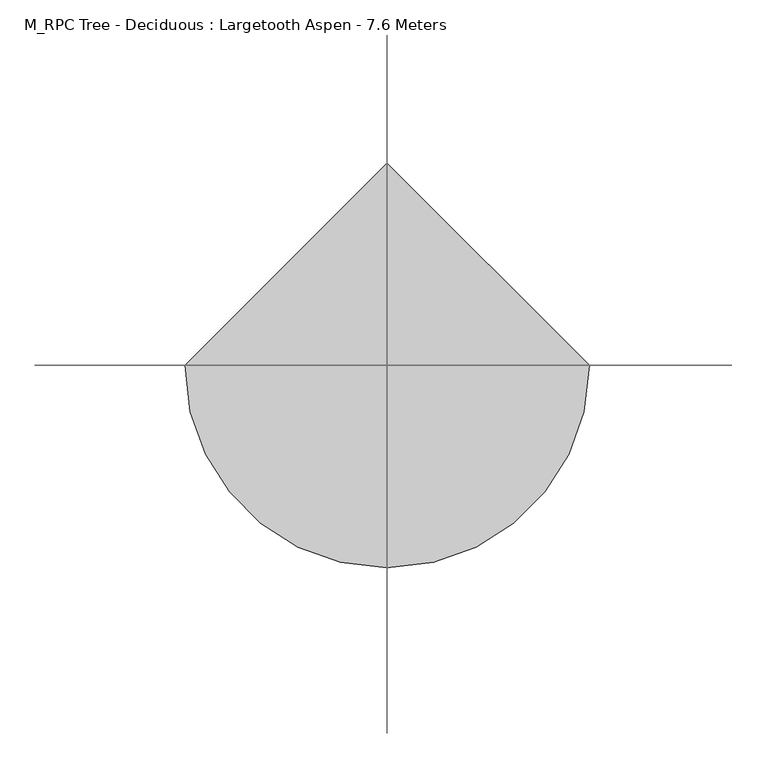
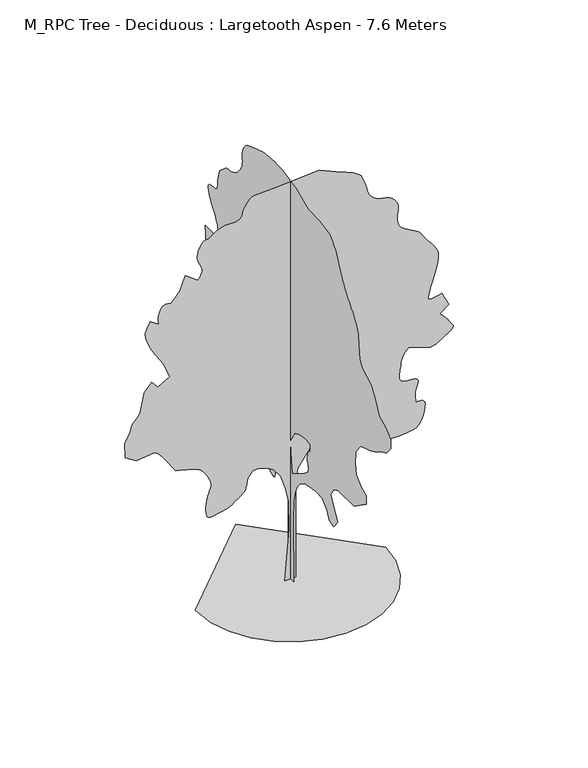
"""IFC4 building model written with IfcOpenShell, lengths in millimetres: geographic element geometry, M_RPC Tree - Deciduous : Largetooth Aspen - 7.6 Meters."""

from ifc_helpers import new_model, si_unit, origin, place, context, project, spatial, triangles, source, transform, mapped, element, save


def m_rpc_tree_deciduous_largetooth_aspen_7_6_meters_a2efc43f(model_context):
    return source(origin(), model_context, "Body", "Tessellation", [
        triangles([(92.8617737, 0.000406, 0.005513), (-103.915959, 0.000406, 0.005513), (-22.8901635, 0.0003494, 949.1680813), (-34.4652064, 0.0003176, 1481.626133), (-92.3406663, 0.0003011, 1759.4311237), (-173.3674883, 0.0002866, 2002.5093098), (-300.6936918, 0.0002762, 2176.1362118), (-404.8693279, 0.0002728, 2234.0127663), (-566.9214277, 0.0002694, 2291.8891754), (-682.6743914, 0.0002694, 2291.8891754), (-763.7004049, 0.0002762, 2176.1362118), (-798.427355, 0.0002852, 2025.6589142), (-801.2950579, 0.0002863, 2008.1460297), (-806.4934324, 0.0002874, 1989.7185207), (-816.3455927, 0.0002886, 1969.4722275), (-833.1871519, 0.0002899, 1946.489764), (-859.3387533, 0.0002915, 1919.8644997), (-897.1360102, 0.0002934, 1888.6816647), (-948.9046526, 0.0002956, 1852.0320122), (-998.3097038, 0.0002977, 1817.003627), (-1032.3247061, 0.0002993, 1790.0718407), (-1058.2431822, 0.0003005, 1769.4200489), (-1083.3510246, 0.0003015, 1753.2219097), (-1114.9365967, 0.0003023, 1739.6560226), (-1160.2933485, 0.000303, 1726.8980804), (-1226.7072453, 0.0003038, 1713.1294441), (-1299.8367931, 0.0003048, 1697.5064152), (-1361.0192505, 0.0003056, 1683.0943588), (-1411.0653236, 0.0003062, 1673.9514576), (-1450.7852829, 0.0003062, 1674.1187439), (-1480.9902706, 0.0003054, 1687.6517841), (-1502.4856155, 0.0003035, 1718.5964069), (-1516.0869656, 0.0003004, 1771.0059986), (-1522.0251205, 0.0002967, 1833.4043701), (-1521.0802654, 0.0002932, 1891.7521168), (-1514.8710514, 0.00029, 1946.2541679), (-1505.0164204, 0.0002869, 1997.1108021), (-1493.1376396, 0.0002841, 2044.5246231), (-1480.8535057, 0.0002815, 2088.6983803), (-1469.7852859, 0.000279, 2129.8370029), (-1458.1775642, 0.0002769, 2165.8103886), (-1444.9485752, 0.000275, 2196.5194153), (-1432.7328964, 0.0002733, 2225.2042923), (-1424.1600185, 0.0002715, 2255.1052288), (-1421.8648098, 0.0002695, 2289.4596725), (-1428.479377, 0.000267, 2331.5079781), (-1446.6356815, 0.0002638, 2384.4900639), (-1473.3978561, 0.0002604, 2441.7913628), (-1503.3976238, 0.0002573, 2494.2338013), (-1535.6266159, 0.0002545, 2541.2094223), (-1569.0690514, 0.0002521, 2582.1226227), (-1602.7142361, 0.00025, 2616.3228607), (-1635.5487144, 0.0002484, 2643.2520309), (-1666.5642632, 0.0002473, 2662.3026123), (-1701.7269424, 0.0002464, 2677.1732162), (-1746.6125748, 0.0002455, 2692.0694), (-1799.5946606, 0.0002446, 2706.940004), (-1859.0568741, 0.0002437, 2721.8358971), (-1923.3782387, 0.0002428, 2736.706501), (-1990.9396671, 0.000242, 2751.5771049), (-2060.1197468, 0.0002411, 2766.4732887), (-2256.8962532, 0.0002238, 3055.8556252), (-2301.7818855, 0.0002202, 3116.5289566), (-2338.160479, 0.0002175, 3161.4195305), (-2367.4508423, 0.0002156, 3193.1367805), (-2391.0741096, 0.0002144, 3214.3154297), (-2410.4440029, 0.0002136, 3227.61549), (-2426.9815109, 0.0002131, 3235.6461044), (-2442.1003555, 0.0002128, 3241.041996), (-2766.1945267, 0.0002148, 3206.3353935), (-2962.9836777, 0.0002073, 3333.6607613), (-2974.5611687, 0.0001914, 3599.8884064), (-2952.3436295, 0.000189, 3639.5351143), (-2930.8609291, 0.0001867, 3678.9789276), (-2910.7717484, 0.0001843, 3718.0428223), (-2892.8103447, 0.0001821, 3756.473616), (-2877.7118477, 0.0001798, 3794.0934128), (-2866.1343567, 0.0001776, 3830.70019), (-2858.8130013, 0.0001755, 3866.1160515), (-2847.3878265, 0.0001735, 3899.5814507), (-2825.6772331, 0.0001716, 3931.2481224), (-2797.4559906, 0.0001698, 3962.0787987), (-2766.6000252, 0.0001679, 3993.137368), (-2736.9852631, 0.000166, 4025.3865623), (-2712.4120537, 0.000164, 4059.8905609), (-2696.7560326, 0.0001617, 4097.611805), (-2627.2919586, 0.000141, 4444.881015), (-2488.4021805, 0.0001321, 4595.3354942), (-2384.2239464, 0.0001396, 4468.0101265), (-2164.2953648, 0.0001327, 4583.7832924), (-2280.0483284, 0.0001155, 4873.1403397), (-2465.2501053, 9.82e-05, 5162.5226761), (-2487.5231644, 9.58e-05, 5203.6643509), (-2513.036142, 9.27e-05, 5254.9385468), (-2539.3601166, 8.93e-05, 5312.268187), (-2564.0600624, 8.58e-05, 5371.6238663), (-2584.7067673, 8.24e-05, 5428.9535065), (-2598.8934013, 7.93e-05, 5480.2277023), (-2604.1628471, 7.69e-05, 5521.3693771), (-2601.4519661, 7.48e-05, 5555.7463486), (-2593.9027176, 7.28e-05, 5589.5407974), (-2582.2746483, 7.08e-05, 5622.8038834), (-2567.4293335, 6.89e-05, 5655.6611801), (-2550.1521904, 6.69e-05, 5688.2394241), (-2531.2585762, 6.5e-05, 5720.5903564), (-2511.5516396, 6.31e-05, 5752.8651306), (-2361.0744873, 6.93e-05, 5648.6941635), (-2365.8675087, 6.73e-05, 5681.019516), (-2369.6472198, 6.54e-05, 5713.8518143), (-2371.4003105, 6.34e-05, 5747.6968414), (-2370.118412, 6.13e-05, 5783.0621246), (-2364.7857433, 5.9e-05, 5820.4540283), (-2354.391465, 5.67e-05, 5860.3794983), (-2337.9248829, 5.41e-05, 5903.344899), (-2316.394075, 5.19e-05, 5940.9141174), (-2291.8258072, 5.04e-05, 5965.7155106), (-2264.7267345, 4.95e-05, 5979.8768555), (-2235.6036575, 4.92e-05, 5985.5515091), (-2204.9604698, 4.92e-05, 5984.8422501), (-2173.3064426, 4.95e-05, 5979.8768555), (-2141.1459057, 5e-05, 5972.7831024), (-1990.6686081, 3.96e-05, 6146.4178528), (-1886.4928448, 2.44e-05, 6401.0680069), (-1666.5642632, 3.41e-05, 6239.0110382), (-1644.4939533, 3.23e-05, 6268.8284042), (-1623.9409927, 3.05e-05, 6298.823085), (-1606.4256374, 2.87e-05, 6329.2229736), (-1593.4675621, 2.69e-05, 6360.2309647), (-1586.584552, 2.5e-05, 6392.0749512), (-1587.2913403, 2.3e-05, 6424.9066681), (-1597.1131245, 2.1e-05, 6458.9545898), (-1613.1085144, 1.89e-05, 6493.7879288), (-1630.1173599, 1.68e-05, 6529.2043716), (-1646.3153538, 1.46e-05, 6565.8614365), (-1659.8813862, 1.23e-05, 6604.3428085), (-1668.993766, 9.9e-06, 6645.2304291), (-1671.8286221, 7.3e-06, 6689.1585617), (-1666.5642632, 4.4e-06, 6736.759726), (-1653.9432312, 1.5e-06, 6785.3747818), (-1636.4607227, -1.2e-06, 6830.974324), (-1614.9299149, -3.6e-06, 6871.9131042), (-1590.1616592, -5.7e-06, 6906.5691284), (-1562.9612846, -7.3e-06, 6933.3209839), (-1534.1394974, -8.3e-06, 6950.5728378), (-1504.512236, -8.7e-06, 6956.6782791), (-1471.3382435, -9.2e-06, 6965.0132355), (-1431.8891979, -1.05e-05, 6986.521225), (-1386.9707188, -1.22e-05, 7015.9078033), (-1337.3959831, -1.41e-05, 7047.9291046), (-1283.9756973, -1.59e-05, 7077.315683), (-1227.5178062, -1.72e-05, 7098.8236725), (-1168.8306908, -1.77e-05, 7107.1580475), (-1109.0314339, -1.76e-05, 7106.8289978), (-1050.4481638, -1.77e-05, 7107.2847839), (-995.7104439, -1.79e-05, 7110.8060806), (-947.4530697, -1.84e-05, 7119.5718246), (-908.3054592, -1.94e-05, 7135.8353668), (-880.9024807, -2.09e-05, 7161.8273849), (-867.8760956, -2.32e-05, 7199.7512329), (-856.9422426, -2.61e-05, 7248.5941818), (-835.6824938, -2.93e-05, 7302.6804153), (-806.5264246, -3.26e-05, 7357.4009125), (-771.9008492, -3.56e-05, 7408.0420074), (-734.2403572, -3.81e-05, 7449.9940979), (-695.9718355, -3.98e-05, 7478.5696793), (-659.5247869, -4.04e-05, 7489.1335693), (-323.8458215, -4.18e-05, 7512.2885513), (509.5693688, -4.53e-05, 7570.1751343), (926.2744205, -3.42e-05, 7384.9631836), (995.3532709, -3.26e-05, 7357.5526474), (1062.2078384, -3.09e-05, 7329.4578506), (1124.6038118, -2.92e-05, 7299.9195374), (1180.3219225, -2.73e-05, 7268.2778641), (1227.1277138, -2.52e-05, 7233.7741562), (1262.7970482, -2.29e-05, 7195.7485703), (1285.1055702, -2.04e-05, 7153.4674301), (1299.9533558, -1.79e-05, 7111.9461273), (1314.5985374, -1.58e-05, 7075.1117477), (1328.8409821, -1.37e-05, 7040.480722), (1342.4753242, -1.16e-05, 7005.6473831), (1355.2991055, -9.4e-06, 6968.1799026), (1367.1094311, -6.8e-06, 6925.6702881), (1377.7063133, -3.9e-06, 6875.662294), (1393.5345623, -8e-07, 6823.9573105), (1419.2834267, 2e-06, 6778.1292938), (1452.117905, 4.3e-06, 6738.3811386), (1489.2059029, 6.3e-06, 6704.890741), (1527.709948, 7.9e-06, 6677.9104111), (1564.7979458, 9.1e-06, 6657.5936279), (1597.6348949, 9.9e-06, 6644.1415421), (1628.0070236, 1.04e-05, 6636.0856384), (1659.1872425, 1.07e-05, 6630.6638763), (1690.5726814, 1.1e-05, 6626.230426), (1721.5527672, 1.13e-05, 6621.2144531), (1751.5195427, 1.17e-05, 6613.9439667), (1779.8675217, 1.24e-05, 6602.8481323), (1805.9861309, 1.34e-05, 6586.2799576), (1831.2638031, 1.47e-05, 6563.7586578), (1856.5388592, 1.63e-05, 6536.6015945), (1880.3977226, 1.82e-05, 6505.7959167), (1901.4218754, 2.02e-05, 6472.3560974), (1918.1949795, 2.23e-05, 6437.2948654), (1929.2986622, 2.44e-05, 6401.625531), (1933.3139694, 2.65e-05, 6366.3364059), (1929.8053173, 2.9e-05, 6325.1191544), (1922.2457497, 3.2e-05, 6273.1351181), (1915.0916805, 3.56e-05, 6213.8805954), (1912.7964718, 3.93e-05, 6150.775145), (1919.8163921, 4.31e-05, 6087.2644867), (1940.6048035, 4.67e-05, 6026.7937592), (1979.615649, 5e-05, 5972.7831024), (2034.2165314, 5.26e-05, 5927.5631882), (2096.1082478, 5.5e-05, 5888.8289246), (2161.2401733, 5.71e-05, 5853.1340103), (2225.5615379, 5.92e-05, 5817.0088898), (2285.0238968, 6.16e-05, 5777.0584213), (2335.5764797, 6.44e-05, 5729.8118866), (2373.1711327, 6.79e-05, 5671.8491455), (2411.6421856, 7.17e-05, 5607.223439), (2462.6659607, 7.56e-05, 5541.7878983), (2518.9567108, 7.96e-05, 5474.7303635), (2573.2307236, 8.38e-05, 5405.2410004), (2618.1721664, 8.81e-05, 5332.5093933), (2646.5201454, 9.27e-05, 5255.7495438), (2650.9785942, 9.76e-05, 5174.0998764), (2634.6386032, 0.0001032, 5079.7841217), (2608.190799, 0.0001097, 4970.8762344), (2575.6628426, 0.0001165, 4855.508567), (2541.0826859, 0.0001233, 4741.7367325), (2508.5622871, 0.0001295, 4637.6927925), (2482.1043091, 0.0001347, 4551.4835197), (2465.7718758, 0.0001383, 4491.1648178), (2464.9611694, 0.0001404, 4454.9635391), (2480.5538223, 0.0001417, 4433.9369156), (2509.8113388, 0.0001422, 4425.5769608), (2550.0001648, 0.0001421, 4427.3248192), (2598.3867462, 0.0001415, 4436.6727951), (2652.2453773, 0.0001407, 4451.0876129), (2708.839888, 0.0001396, 4468.0101265), (2836.1652557, 0.0001548, 4213.3596817), (2674.1332855, 0.0001624, 4086.0346046), (2698.8841003, 0.0001637, 4063.6400414), (2723.4573097, 0.0001651, 4040.7132431), (2747.6253113, 0.0001665, 4016.7987144), (2771.1852104, 0.0001681, 3991.3386406), (2793.9344032, 0.0001697, 3963.8772354), (2815.6705765, 0.0001715, 3933.8828453), (2836.1652557, 0.0001735, 3900.8482338), (2858.1037422, 0.0001754, 3868.6749069), (2881.2584335, 0.000177, 3840.554821), (2901.1702995, 0.0001786, 3814.8921432), (2913.3811821, 0.0001801, 3790.0148827), (2913.4570496, 0.0001816, 3764.3269157), (2896.9144547, 0.0001833, 3736.232119), (2859.3199471, 0.0001852, 3704.0590828), (2604.6695023, 0.0001955, 3530.4243324), (2500.4962097, 0.0001962, 3518.8471321), (2118.5182171, 0.0001886, 3646.1722092), (2091.3836815, 0.0001903, 3618.7110947), (2065.163625, 0.000192, 3590.1349319), (2040.7651142, 0.0001938, 3559.3298355), (2019.0975414, 0.0001958, 3525.1551773), (2001.0780018, 0.0001981, 3486.5726486), (1987.6134167, 0.0002008, 3442.3913338), (1979.615649, 0.0002038, 3391.5220551), (1974.0473843, 0.0002068, 3342.1474525), (1967.6684132, 0.0002092, 3301.2848305), (1961.0868382, 0.0002113, 3266.096862), (1954.9106163, 0.0002132, 3233.7206406), (1949.7477047, 0.0002151, 3201.3699989), (1946.2035896, 0.0002172, 3166.1567413), (1944.888699, 0.0002197, 3125.2941193), (1953.8643139, 0.000222, 3086.7368797), (1977.0163891, 0.0002236, 3059.0981598), (2008.6704163, 0.0002247, 3040.5542336), (2043.1591541, 0.0002254, 3029.3316628), (2074.8131813, 0.0002257, 3023.5555618), (2097.9652565, 0.0002259, 3021.4277847), (2106.9408714, 0.0002259, 3021.1237335), (2119.5973663, 0.0002258, 3022.0103073), (2151.4868443, 0.0002258, 3022.4663841), (2193.5021576, 0.000226, 3019.2997169), (2236.5307812, 0.0002266, 3009.2421913), (2271.4578644, 0.0002278, 2989.0771431), (2289.1759689, 0.0002298, 2955.5102966), (2280.5702442, 0.0002328, 2905.3758568), (2259.8146797, 0.0002362, 2847.8691925), (2246.3499493, 0.0002394, 2794.0105614), (2238.9578133, 0.0002425, 2743.191861), (2236.4270084, 0.0002453, 2694.7799904), (2237.5416206, 0.0002481, 2648.2174255), (2241.0857357, 0.0002508, 2602.8707748), (2245.8432941, 0.0002535, 2558.1066467), (2285.1910378, 0.0002532, 2562.540097), (2322.5171024, 0.0002531, 2563.730722), (2355.7899261, 0.0002535, 2558.4106979), (2382.9903008, 0.0002544, 2543.4133575), (2402.0916058, 0.000256, 2515.4278564), (2411.0672207, 0.0002587, 2471.2540993), (2407.8954666, 0.0002625, 2407.6395229), (2395.1731327, 0.0002668, 2334.9507912), (2376.9836906, 0.0002708, 2266.9155544), (2353.5301804, 0.0002745, 2205.3632069), (2325.0124443, 0.0002777, 2152.110062), (2291.6383186, 0.0002803, 2108.9801365), (2253.6054657, 0.0002821, 2077.7999176), (2211.1189602, 0.0002832, 2060.3858643), (2171.2620907, 0.0002837, 2051.7801395), (2137.4826118, 0.000284, 2045.4011684), (2104.5113686, 0.0002843, 2040.64361), (2067.0864727, 0.0002845, 2036.8967457), (2019.9412399, 0.0002847, 2033.5578506), (1957.8137821, 0.000285, 2030.0137356), (1875.4374149, 0.0002852, 2025.6589142), (1785.9069786, 0.0002851, 2027.1105698), (1704.880965, 0.0002844, 2040.1039627), (1630.9405655, 0.000283, 2062.7139198), (1562.6724941, 0.0002812, 2093.0175934), (1498.6551807, 0.0002791, 2129.0947517), (1437.4727234, 0.0002767, 2169.0176056), (1377.7063133, 0.0002742, 2210.8631618), (1123.0508543, 0.0002597, 2453.9412025), (856.8231365, 0.0002528, 2569.6841377), (544.2937391, 0.0002542, 2546.5547356), (393.8164052, 0.0002611, 2430.7917435), (289.6407691, 0.00027, 2280.3144459), (127.5871523, 0.0002838, 2048.8109894), (92.8617737, 0.0003011, 1759.4311237), (92.8617737, 0.0003383, 1134.3723289), (-0.0023646, 90.6053344, 1.1e-05), (-0.0023646, -94.5971056, 0.0), (-0.0023646, -83.0220672, 1157.5168465), (-0.0023646, -94.5971056, 1527.9227257), (-0.0023646, -140.8980313, 1724.6992321), (-0.0023646, -210.3490428, 1875.1765297), (-0.0023646, -302.9508941, 1990.9294933), (-0.0023646, -441.8534077, 2071.9555069), (-0.0023646, -557.6038279, 2095.1051113), (-0.0023646, -789.1072117, 2141.4067909), (-0.0023646, -985.8861889, 2129.8320614), (-0.0023646, -1136.3635592, 1979.3546185), (-0.0023646, -1205.8147705, 1840.4521957), (-0.0023646, -1333.1399929, 1794.1505161), (-0.0023646, -1472.042561, 1967.7774181), (-0.0023646, -1321.5652634, 2199.2832001), (-0.0023646, -1252.1139793, 2361.3353725), (-0.0023646, -1333.1399929, 2500.2354698), (-0.0023646, -1483.6172905, 2569.6841377), (-0.0023646, -1969.7736626, 2569.6841377), (-0.0023646, -2351.7542713, 2835.9117828), (-0.0023646, -2351.7542713, 2997.9690422), (-0.0023646, -2189.7022442, 3067.4075363), (-0.0023646, -2039.2249466, 3206.3101044), (-0.0023646, -2004.5004673, 3403.0992554), (-0.0023646, -2027.6500717, 3634.5950089), (-0.0023646, -2178.1273693, 3831.3841599), (-0.0023646, -2444.3551598, 3923.9773453), (-0.0023646, -2488.9367409, 3941.4068047), (-0.0023646, -2533.110498, 3959.1147354), (-0.0023646, -2576.4735489, 3977.4307686), (-0.0023646, -2618.6279526, 3996.6839539), (-0.0023646, -2659.1612343, 4017.1280548), (-0.0023646, -2697.6678955, 4039.0918304), (-0.0023646, -2733.7427284, 4062.8799133), (-0.0023646, -2768.4493309, 4086.3386559), (-0.0023646, -2803.1812225, 4107.3652794), (-0.0023646, -2837.9131142, 4126.3652824), (-0.0023646, -2872.6450058, 4143.7438728), (-0.0023646, -2907.351899, 4159.9065491), (-0.0023646, -2942.0837906, 4175.258519), (-0.0023646, -2976.8156822, 4190.2052811), (-0.0023646, -3104.1407593, 4352.2622498), (-0.0023646, -3104.1407593, 4514.3195091), (-0.0023646, -2953.6609909, 4653.2220772), (-0.0023646, -2756.8971291, 4757.3924629), (-0.0023646, -2629.5467628, 5000.4657074), (-0.0023646, -2502.234185, 5185.6776581), (-0.0023646, -2224.4290489, 5336.1574265), (-0.0023646, -2143.4030354, 5463.4827942), (-0.0023646, -2120.2509602, 5718.1329483), (-0.0023646, -2097.1013557, 5926.4743011), (-0.0023646, -2072.264645, 5978.4327576), (-0.0023646, -2047.225185, 6029.4540619), (-0.0023646, -2021.7779011, 6078.651059), (-0.0023646, -1995.7251308, 6125.1127579), (-0.0023646, -1968.8641251, 6167.9514221), (-0.0023646, -1940.9873383, 6206.2043198), (-0.0023646, -1911.8997242, 6239.0110382), (-0.0023646, -1875.8225658, 6277.7964615), (-0.0023646, -1830.2327614, 6330.9455429), (-0.0023646, -1779.7788643, 6393.0121033), (-0.0023646, -1729.1274502, 6458.4988037), (-0.0023646, -1682.9270725, 6521.9838821), (-0.0023646, -1645.83922, 6577.9705811), (-0.0023646, -1622.5198586, 6620.9865601), (-0.0023646, -1605.6807701, 6657.1372604), (-0.0023646, -1585.6016178, 6696.1255783), (-0.0023646, -1563.2930958, 6737.9253525), (-0.0023646, -1539.7736012, 6782.5877426), (-0.0023646, -1516.0490318, 6830.0627518), (-0.0023646, -1493.1350235, 6880.3742157), (-0.0023646, -1472.042561, 6933.5238785), (-0.0023646, -1448.8245014, 6986.749118), (-0.0023646, -1419.5316673, 7037.5425293), (-0.0023646, -1385.1770782, 7086.3087387), (-0.0023646, -1346.7743351, 7133.4541168), (-0.0023646, -1305.3316612, 7179.3832901), (-0.0023646, -1261.8673084, 7224.5020477), (-0.0023646, -1217.3895727, 7269.2155975), (-0.0023646, -893.2828297, 7327.0766006), (-0.0023646, -546.029062, 7338.653801), (-0.0023646, -175.623419, 7500.711351), (-0.0023646, 264.2314734, 7593.3045364), (-0.0023646, 323.6937959, 7595.7363647), (-0.0023646, 382.7508016, 7597.8641418), (-0.0023646, 440.9996807, 7599.3843979), (-0.0023646, 498.0300296, 7599.9925003), (-0.0023646, 553.4441254, 7599.3843979), (-0.0023646, 606.831528, 7597.2566208), (-0.0023646, 657.7895004, 7593.3045364), (-0.0023646, 706.7891258, 7588.2379852), (-0.0023646, 754.9781902, 7582.5883301), (-0.0023646, 802.9670488, 7575.6974716), (-0.0023646, 851.3612606, 7566.9828873), (-0.0023646, 900.7663118, 7555.8620544), (-0.0023646, 951.7900869, 7541.6751297), (-0.0023646, 1005.0432318, 7523.8657516), (-0.0023646, 1340.7248497, 7408.1181656), (-0.0023646, 1370.3545818, 7383.1138779), (-0.0023646, 1399.173753, 7356.8683868), (-0.0023646, 1426.3741276, 7328.2166473), (-0.0023646, 1451.1425285, 7295.9418732), (-0.0023646, 1472.6733364, 7258.7778625), (-0.0023646, 1490.1558449, 7215.5595703), (-0.0023646, 1502.7768768, 7165.019632), (-0.0023646, 1507.1292274, 7116.7342072), (-0.0023646, 1503.584967, 7077.7714691), (-0.0023646, 1497.0060081, 7043.2421814), (-0.0023646, 1492.2458336, 7008.3076859), (-0.0023646, 1494.1711521, 6968.128743), (-0.0023646, 1507.6358826, 6917.7916992), (-0.0023646, 1537.5012108, 6852.5078934), (-0.0023646, 1578.4019119, 6786.1851974), (-0.0023646, 1620.9238804, 6734.4546341), (-0.0023646, 1663.8485859, 6694.8587952), (-0.0023646, 1705.9652012, 6664.9908508), (-0.0023646, 1746.0576668, 6642.4189728), (-0.0023646, 1782.9075977, 6624.7107513), (-0.0023646, 1815.3063469, 6609.4093597), (-0.0023646, 1845.0703732, 6598.3135254), (-0.0023646, 1874.8345448, 6592.8923447), (-0.0023646, 1904.598571, 6590.2826202), (-0.0023646, 1934.3652134, 6587.6984756), (-0.0023646, 1964.129385, 6582.2522964), (-0.0023646, 1993.8934113, 6571.1558807), (-0.0023646, 2023.6575829, 6551.5483566), (-0.0023646, 2197.2869556, 6401.0680069), (-0.0023646, 2266.7357689, 6181.1500351), (-0.0023646, 2264.4760231, 6146.5445892), (-0.0023646, 2263.5310226, 6112.7751389), (-0.0023646, 2265.2182743, 6080.6021027), (-0.0023646, 2270.8549942, 6050.8858932), (-0.0023646, 2281.7533115, 6024.3875107), (-0.0023646, 2299.23582, 6001.9417877), (-0.0023646, 2324.612178, 5984.3608841), (-0.0023646, 2359.9116222, 5974.3033585), (-0.0023646, 2402.9047829, 5970.5285889), (-0.0023646, 2448.5301956, 5967.9700241), (-0.0023646, 2491.7284309, 5961.5605316), (-0.0023646, 2527.4306122, 5946.2341415), (-0.0023646, 2550.5826874, 5916.92314), (-0.0023646, 2556.1053154, 5868.6127167), (-0.0023646, 2547.4413094, 5812.448703), (-0.0023646, 2532.0893394, 5762.3651321), (-0.0023646, 2511.1641632, 5717.3475311), (-0.0023646, 2485.7878052, 5676.3837524), (-0.0023646, 2457.0700813, 5638.4599045), (-0.0023646, 2426.1228424, 5602.562677), (-0.0023646, 2394.0634621, 5567.6531799), (-0.0023646, 2369.3609001, 5525.4981949), (-0.0023646, 2345.2664406, 5483.4705276), (-0.0023646, 2322.3854244, 5441.6201752), (-0.0023646, 2301.3284248, 5400.0732925), (-0.0023646, 2282.698312, 5358.9321991), (-0.0023646, 2267.1081299, 5318.2974701), (-0.0023646, 2255.160894, 5278.2708435), (-0.0023646, 2248.95168, 5240.6254669), (-0.0023646, 2249.4254883, 5206.6025436), (-0.0023646, 2255.4649452, 5175.6201324), (-0.0023646, 2265.9605255, 5147.0695496), (-0.0023646, 2279.797617, 5120.3426926), (-0.0023646, 2295.861462, 5094.8320404), (-0.0023646, 2313.0374485, 5069.9294907), (-0.0023646, 2463.5147461, 5093.0844727), (-0.0023646, 2648.7240807, 5093.0844727), (-0.0023646, 2625.5693893, 4757.3924629), (-0.0023646, 2417.2130665, 4398.5716324), (-0.0023646, 2409.7574169, 4356.4422272), (-0.0023646, 2402.1979946, 4314.642453), (-0.0023646, 2394.4358231, 4273.4252014), (-0.0023646, 2386.3697456, 4233.1451019), (-0.0023646, 2377.898315, 4194.0559181), (-0.0023646, 2368.9227001, 4156.486409), (-0.0023646, 2359.3391281, 4120.7664963), (-0.0023646, 2344.9953815, 4082.1586784), (-0.0023646, 2323.9712288, 4037.2681046), (-0.0023646, 2299.5044083, 3988.3492882), (-0.0023646, 2274.8373093, 3937.5814568), (-0.0023646, 2253.2051994, 3887.2441223), (-0.0023646, 2237.8507587, 3839.5162216), (-0.0023646, 2232.0114349, 3796.6522682), (-0.0023646, 2236.7360012, 3758.6522621), (-0.0023646, 2249.9651356, 3723.6921867), (-0.0023646, 2270.279884, 3691.2656776), (-0.0023646, 2296.2641991, 3660.865789), (-0.0023646, 2326.5020336, 3631.9602859), (-0.0023646, 2359.5747242, 3604.0936729), (-0.0023646, 2394.0634621, 3576.7337151), (-0.0023646, 2706.5853745, 3646.1722092), (-0.0023646, 2723.8372284, 3596.6458717), (-0.0023646, 2740.3798233, 3547.4991623), (-0.0023646, 2755.5039001, 3499.1884483), (-0.0023646, 2768.4746201, 3452.0686501), (-0.0023646, 2778.6333023, 3406.5699738), (-0.0023646, 2785.245108, 3363.0979179), (-0.0023646, 2787.6266487, 3322.0832703), (-0.0023646, 2774.199852, 3282.9940865), (-0.0023646, 2739.6958534, 3244.7153183), (-0.0023646, 2692.8545265, 3206.6647339), (-0.0023646, 2642.3654572, 3168.1833618), (-0.0023646, 2596.9426483, 3128.7142593), (-0.0023646, 2565.3015564, 3087.5981644), (-0.0023646, 2556.1053154, 3044.2784248), (-0.0023646, 2564.4399811, 3002.6556747), (-0.0023646, 2578.8547989, 2966.5049744), (-0.0023646, 2598.3361679, 2934.9397499), (-0.0023646, 2621.8454887, 2906.9969788), (-0.0023646, 2648.4200294, 2881.7903778), (-0.0023646, 2676.9959015, 2858.3825043), (-0.0023646, 2706.5853745, 2835.9117828), (-0.0023646, 2776.0491577, 2604.4160294), (-0.0023646, 2709.3974121, 2602.1106468), (-0.0023646, 2644.670549, 2600.945311), (-0.0023646, 2583.7946136, 2601.984201), (-0.0023646, 2528.6796638, 2606.3667824), (-0.0023646, 2481.2656975, 2615.2081032), (-0.0023646, 2443.468586, 2629.6226303), (-0.0023646, 2417.2130665, 2650.725412), (-0.0023646, 2391.9710026, 2676.8694557), (-0.0023646, 2357.0109272, 2705.4453278), (-0.0023646, 2313.9494568, 2736.0478203), (-0.0023646, 2264.407568, 2768.2973053), (-0.0023646, 2210.0068188, 2801.7371246), (-0.0023646, 2152.3684765, 2835.987941), (-0.0023646, 2093.1088669, 2870.6436745), (-0.0023646, 2090.6463718, 2833.3785072), (-0.0023646, 2088.2828533, 2795.8345779), (-0.0023646, 2086.1244095, 2757.6572571), (-0.0023646, 2084.2675461, 2718.5680733), (-0.0023646, 2082.8158905, 2678.2879738), (-0.0023646, 2081.8710354, 2636.4626198), (-0.0023646, 2081.533992, 2592.838829), (-0.0023646, 2079.9481876, 2547.390731), (-0.0023646, 2074.514217, 2502.7332825), (-0.0023646, 2064.2212406, 2462.5418404), (-0.0023646, 2048.0560936, 2430.4471424), (-0.0023646, 2025.0077911, 2410.0994019), (-0.0023646, 1994.0631683, 2405.1366234), (-0.0023646, 1954.2062988, 2419.2093109), (-0.0023646, 1909.2219807, 2445.3635284), (-0.0023646, 1863.6321762, 2473.9469582), (-0.0023646, 1817.5331005, 2504.5546829), (-0.0023646, 1771.028817, 2536.7762627), (-0.0023646, 1724.222953, 2570.216082), (-0.0023646, 1677.2144852, 2604.4921875), (-0.0023646, 1630.1020992, 2639.147921), (-0.0023646, 1352.2995792, 2720.1639061), (-0.0023646, 1074.4945158, 2627.5707207), (-0.0023646, 900.8676138, 2419.2093109), (-0.0023646, 923.2419748, 2389.5794334), (-0.0023646, 945.9203871, 2360.7602623), (-0.0023646, 969.204213, 2333.5598877), (-0.0023646, 993.4000471, 2308.7914867), (-0.0023646, 1018.8119408, 2287.2608242), (-0.0023646, 1045.7412563, 2269.7783157), (-0.0023646, 1074.4945158, 2257.1571384), (-0.0023646, 1101.897567, 2244.8731499), (-0.0023646, 1125.0471714, 2228.3379673), (-0.0023646, 1144.6551315, 2208.258815), (-0.0023646, 1161.4257648, 2185.344952), (-0.0023646, 1176.07349, 2160.305492), (-0.0023646, 1189.3025517, 2133.8473686), (-0.0023646, 1201.8222816, 2106.6798409), (-0.0023646, 1169.4919149, 2099.1888737), (-0.0023646, 1136.6573639, 2091.3937099), (-0.0023646, 1102.8070318, 2082.9907345), (-0.0023646, 1067.4417486, 2073.6756054), (-0.0023646, 1030.0497723, 2063.1471783), (-0.0023646, 990.1269911, 2051.0986404), (-0.0023646, 947.16675, 2037.2285568), (-0.0023646, 904.2091249, 2020.3237747), (-0.0023646, 864.2863438, 1999.7708141), (-0.0023646, 826.8943674, 1976.1830097), (-0.0023646, 791.5265408, 1950.1630863), (-0.0023646, 757.6786795, 1922.3217625), (-0.0023646, 724.8442011, 1893.2645245), (-0.0023646, 692.5138344, 1863.6018002), (-0.0023646, 692.5138344, 1701.5496277), (-0.0023646, 650.5998957, 1674.7216141), (-0.0023646, 610.2059223, 1650.6246838), (-0.0023646, 572.8469018, 1631.9970417), (-0.0023646, 540.0453429, 1621.5699165), (-0.0023646, 513.3187039, 1622.0765717), (-0.0023646, 494.1844431, 1636.2505611), (-0.0023646, 484.160055, 1666.8252937), (-0.0023646, 479.2682024, 1701.4811726), (-0.0023646, 474.7791232, 1728.6487003), (-0.0023646, 471.100714, 1752.1706657), (-0.0023646, 468.638328, 1775.8927643), (-0.0023646, 467.7947385, 1803.6682491), (-0.0023646, 468.9752624, 1839.3374382), (-0.0023646, 472.5852528, 1886.7512592), (-0.0023646, 475.5213744, 1938.6212036), (-0.0023646, 474.8120427, 1985.6298168), (-0.0023646, 471.0677945, 2028.5899853), (-0.0023646, 464.8915363, 2068.3100899), (-0.0023646, 456.893805, 2105.6006916), (-0.0023646, 447.6800869, 2141.2724968), (-0.0023646, 437.8608825, 2176.1311249), (-0.0023646, 241.0823958, 2187.7059998), (-0.0023646, 136.90626, 1990.9294933), (-0.0023646, 79.030296, 1655.2479481), (-0.0023646, 79.030296, 1226.9681305), (-0.0023646, 79.030296, 590.3344608), (-0.0022449, -48.2969385, 2025.6538273), (-0.0022449, -1.9959556, 2396.0597065), (-0.0022449, 9.5791312, 2615.9935204), (-0.0022449, -129.3229929, 2835.9117828), (-0.0022449, -279.801326, 2905.3758568), (-0.0022449, -453.4282099, 2928.5049683), (-0.0022449, -615.4803097, 2928.5049683), (-0.0022449, -615.4803097, 2789.62798), (-0.0022449, -534.4542598, 2720.1639061), (-0.0022449, -511.3046917, 2558.1066467), (-0.0022449, -521.1568156, 2548.0241226), (-0.0022449, -530.6061298, 2536.9279976), (-0.0022449, -539.2448104, 2523.7927528), (-0.0022449, -546.6699749, 2507.6277512), (-0.0022449, -552.4738358, 2487.4115433), (-0.0022449, -556.2535832, 2462.1366325), (-0.0022449, -557.6038279, 2430.7840405), (-0.0022449, -554.2294335, 2398.4207542), (-0.0022449, -544.7801193, 2370.3109875), (-0.0022449, -530.2691955, 2345.7427197), (-0.0022449, -511.7075014, 2324.0093079), (-0.0022449, -490.1108545, 2304.4038185), (-0.0022449, -466.4875508, 2286.2145218), (-0.0022449, -441.8534077, 2268.7320133), (-1707.3661331, 0.0, 0.0031185), (-1662.2297894, -391.2146745, 0.0030952), (-1533.678479, -750.4840605, 0.0030738), (-1332.01012, -1067.5126745, 0.0030549), (-1067.5126745, -1332.01012, 0.0030391), (-750.4840605, -1533.678479, 0.0030271), (-391.2146745, -1662.2297894, 0.0030194), (7.48e-05, -1707.3661331, 0.0030167), (391.2146745, -1662.2297894, 0.0030194), (750.4840605, -1533.678479, 0.0030271), (1067.5126745, -1332.01012, 0.0030391), (1332.01012, -1067.5126745, 0.0030549), (1533.678479, -750.4840605, 0.0030738), (1662.2297894, -391.2146745, 0.0030952), (1707.3661331, 0.0001493, 0.0031185), (-0.0002245, 1707.3661331, 0.0032203)], [[122, 123, 124], [87, 88, 89], [1, 2, 3], [329, 1, 3], [329, 3, 4], [328, 329, 4], [328, 4, 5], [105, 106, 107], [327, 328, 5], [327, 5, 6], [104, 105, 107], [238, 239, 240], [238, 240, 241], [237, 238, 241], [236, 237, 241], [103, 104, 107], [86, 87, 89], [235, 236, 241], [102, 103, 107], [101, 102, 107], [100, 101, 107], [99, 100, 107], [98, 99, 107], [97, 98, 107], [96, 97, 107], [327, 6, 7], [326, 327, 7], [95, 96, 107], [70, 71, 72], [69, 70, 72], [69, 72, 73], [69, 73, 74], [69, 74, 75], [69, 75, 76], [69, 76, 77], [69, 77, 78], [94, 95, 107], [234, 235, 241], [93, 94, 107], [69, 78, 79], [69, 79, 80], [69, 80, 81], [69, 81, 82], [69, 82, 83], [69, 83, 84], [69, 84, 85], [68, 69, 85], [325, 326, 7], [325, 7, 8], [67, 68, 85], [92, 93, 107], [91, 92, 107], [60, 61, 62], [67, 85, 86], [67, 86, 89], [67, 89, 90], [66, 67, 90], [65, 66, 90], [64, 65, 90], [63, 64, 90], [62, 63, 90], [60, 62, 90], [59, 60, 90], [58, 59, 90], [57, 58, 90], [56, 57, 90], [55, 56, 90], [54, 55, 90], [53, 54, 90], [284, 285, 286], [283, 284, 286], [282, 283, 286], [282, 286, 287], [281, 282, 287], [280, 281, 287], [279, 280, 287], [279, 287, 288], [278, 279, 288], [277, 278, 288], [277, 288, 289], [276, 277, 289], [275, 276, 289], [275, 289, 290], [52, 53, 90], [325, 8, 9], [121, 122, 124], [275, 290, 291], [30, 31, 32], [29, 30, 32], [29, 32, 33], [28, 29, 33], [28, 33, 34], [27, 28, 34], [27, 34, 35], [27, 35, 36], [26, 27, 36], [26, 36, 37], [26, 37, 38], [25, 26, 38], [25, 38, 39], [24, 25, 39], [23, 24, 39], [22, 23, 39], [21, 22, 39], [20, 21, 39], [20, 39, 40], [20, 40, 41], [20, 41, 42], [19, 20, 42], [19, 42, 43], [18, 19, 43], [18, 43, 44], [17, 18, 44], [16, 17, 44], [15, 16, 44], [14, 15, 44], [13, 14, 44], [12, 13, 44], [11, 12, 44], [11, 44, 45], [11, 45, 46], [10, 11, 46], [10, 46, 47], [10, 47, 48], [10, 48, 49], [10, 49, 50], [10, 50, 51], [252, 253, 254], [251, 252, 254], [251, 254, 255], [250, 251, 255], [249, 250, 255], [249, 255, 256], [248, 249, 256], [247, 248, 256], [246, 247, 256], [245, 246, 256], [245, 256, 257], [245, 257, 258], [244, 245, 258], [243, 244, 258], [242, 243, 258], [241, 242, 258], [234, 241, 258], [233, 234, 258], [274, 275, 291], [324, 325, 9], [51, 52, 90], [10, 51, 90], [9, 10, 90], [324, 9, 90], [323, 324, 90], [323, 90, 91], [323, 91, 107], [323, 107, 108], [323, 108, 109], [323, 109, 110], [323, 110, 111], [323, 111, 112], [323, 112, 113], [323, 113, 114], [323, 114, 115], [323, 115, 116], [323, 116, 117], [323, 117, 118], [323, 118, 119], [323, 119, 120], [323, 120, 121], [323, 121, 124], [323, 124, 125], [323, 125, 126], [323, 126, 127], [323, 127, 128], [323, 128, 129], [322, 323, 129], [322, 129, 130], [167, 168, 169], [274, 291, 292], [296, 297, 298], [296, 298, 299], [295, 296, 299], [294, 295, 299], [294, 299, 300], [293, 294, 300], [293, 300, 301], [293, 301, 302], [293, 302, 303], [293, 303, 304], [293, 304, 305], [293, 305, 306], [293, 306, 307], [293, 307, 308], [293, 308, 309], [293, 309, 310], [293, 310, 311], [293, 311, 312], [293, 312, 313], [293, 313, 314], [293, 314, 315], [293, 315, 316], [293, 316, 317], [293, 317, 318], [293, 318, 319], [292, 293, 319], [274, 292, 319], [274, 319, 320], [274, 320, 321], [274, 321, 322], [273, 274, 322], [273, 322, 130], [272, 273, 130], [271, 272, 130], [270, 271, 130], [269, 270, 130], [268, 269, 130], [267, 268, 130], [266, 267, 130], [265, 266, 130], [264, 265, 130], [263, 264, 130], [262, 263, 130], [261, 262, 130], [260, 261, 130], [259, 260, 130], [258, 259, 130], [233, 258, 130], [232, 233, 130], [231, 232, 130], [230, 231, 130], [229, 230, 130], [228, 229, 130], [227, 228, 130], [226, 227, 130], [225, 226, 130], [224, 225, 130], [223, 224, 130], [222, 223, 130], [221, 222, 130], [220, 221, 130], [219, 220, 130], [218, 219, 130], [217, 218, 130], [216, 217, 130], [215, 216, 130], [214, 215, 130], [213, 214, 130], [212, 213, 130], [211, 212, 130], [210, 211, 130], [209, 210, 130], [208, 209, 130], [207, 208, 130], [206, 207, 130], [205, 206, 130], [204, 205, 130], [203, 204, 130], [202, 203, 130], [201, 202, 130], [200, 201, 130], [199, 200, 130], [198, 199, 130], [197, 198, 130], [196, 197, 130], [195, 196, 130], [194, 195, 130], [193, 194, 130], [192, 193, 130], [191, 192, 130], [190, 191, 130], [189, 190, 130], [188, 189, 130], [187, 188, 130], [186, 187, 130], [185, 186, 130], [184, 185, 130], [183, 184, 130], [182, 183, 130], [181, 182, 130], [180, 181, 130], [179, 180, 130], [178, 179, 130], [177, 178, 130], [176, 177, 130], [175, 176, 130], [174, 175, 130], [173, 174, 130], [172, 173, 130], [171, 172, 130], [170, 171, 130], [169, 170, 130], [167, 169, 130], [167, 130, 131], [167, 131, 132], [167, 132, 133], [167, 133, 134], [167, 134, 135], [167, 135, 136], [164, 165, 166], [164, 166, 167], [163, 164, 167], [162, 163, 167], [161, 162, 167], [160, 161, 167], [159, 160, 167], [158, 159, 167], [143, 144, 145], [142, 143, 145], [141, 142, 145], [140, 141, 145], [140, 145, 146], [139, 140, 146], [138, 139, 146], [137, 138, 146], [136, 137, 146], [136, 146, 147], [136, 147, 148], [136, 148, 149], [136, 149, 150], [136, 150, 151], [136, 151, 152], [136, 152, 153], [136, 153, 154], [136, 154, 155], [136, 155, 156], [157, 158, 167], [157, 167, 136], [157, 136, 156], [634, 330, 635], [633, 634, 635], [632, 633, 635], [631, 632, 635], [540, 541, 542], [592, 593, 594], [494, 495, 496], [635, 330, 331], [635, 331, 332], [635, 332, 333], [635, 333, 334], [635, 334, 335], [658, 635, 335], [658, 335, 336], [658, 336, 337], [658, 337, 338], [540, 542, 543], [657, 658, 338], [631, 635, 636], [630, 631, 636], [518, 519, 520], [656, 657, 338], [656, 338, 339], [655, 656, 339], [654, 655, 339], [653, 654, 339], [540, 543, 544], [539, 540, 544], [518, 520, 521], [539, 544, 545], [538, 539, 545], [538, 545, 546], [538, 546, 547], [538, 547, 548], [537, 538, 548], [537, 548, 549], [536, 537, 549], [536, 549, 550], [536, 550, 551], [535, 536, 551], [535, 551, 552], [534, 535, 552], [493, 494, 496], [493, 496, 497], [343, 344, 345], [342, 343, 345], [341, 342, 345], [340, 341, 345], [340, 345, 346], [534, 552, 553], [533, 534, 553], [518, 521, 522], [350, 351, 352], [349, 350, 352], [349, 352, 353], [348, 349, 353], [533, 553, 554], [652, 653, 339], [518, 522, 523], [518, 523, 524], [533, 554, 555], [532, 533, 555], [518, 524, 525], [518, 525, 526], [518, 526, 527], [518, 527, 528], [518, 528, 529], [518, 529, 530], [518, 530, 531], [518, 531, 532], [518, 532, 555], [517, 518, 555], [516, 517, 555], [515, 516, 555], [607, 608, 609], [591, 592, 594], [591, 594, 595], [590, 591, 595], [590, 595, 596], [589, 590, 596], [588, 589, 596], [588, 596, 597], [587, 588, 597], [586, 587, 597], [586, 597, 598], [585, 586, 598], [585, 598, 599], [584, 585, 599], [584, 599, 600], [583, 584, 600], [583, 600, 601], [582, 583, 601], [514, 515, 555], [643, 644, 645], [630, 636, 637], [629, 630, 637], [581, 582, 601], [581, 601, 602], [348, 353, 354], [580, 581, 602], [580, 602, 603], [579, 580, 603], [651, 652, 339], [651, 339, 340], [651, 340, 346], [650, 651, 346], [649, 650, 346], [649, 346, 347], [648, 649, 347], [647, 648, 347], [646, 647, 347], [372, 373, 374], [371, 372, 374], [370, 371, 374], [369, 370, 374], [369, 374, 375], [368, 369, 375], [367, 368, 375], [366, 367, 375], [365, 366, 375], [364, 365, 375], [363, 364, 375], [362, 363, 375], [361, 362, 375], [360, 361, 375], [359, 360, 375], [358, 359, 375], [357, 358, 375], [356, 357, 375], [356, 375, 376], [356, 376, 377], [356, 377, 378], [645, 646, 347], [643, 645, 347], [642, 643, 347], [641, 642, 347], [641, 347, 348], [641, 348, 354], [641, 354, 355], [607, 609, 610], [513, 514, 555], [579, 603, 604], [607, 610, 611], [607, 611, 612], [607, 612, 613], [607, 613, 614], [607, 614, 615], [607, 615, 616], [607, 616, 617], [607, 617, 618], [607, 618, 619], [607, 619, 620], [607, 620, 621], [607, 621, 622], [607, 622, 623], [607, 623, 624], [606, 607, 624], [606, 624, 625], [605, 606, 625], [605, 625, 626], [604, 605, 626], [579, 604, 626], [579, 626, 627], [579, 627, 628], [579, 628, 629], [579, 629, 637], [578, 579, 637], [578, 637, 638], [355, 356, 378], [641, 355, 378], [641, 378, 379], [640, 641, 379], [639, 640, 379], [639, 379, 380], [639, 380, 381], [639, 381, 382], [639, 382, 383], [639, 383, 384], [639, 384, 385], [639, 385, 386], [639, 386, 387], [639, 387, 388], [639, 388, 389], [639, 389, 390], [639, 390, 391], [639, 391, 392], [639, 392, 393], [639, 393, 394], [639, 394, 395], [638, 639, 395], [578, 638, 395], [577, 578, 395], [577, 395, 396], [577, 396, 397], [577, 397, 398], [577, 398, 399], [577, 399, 400], [577, 400, 401], [577, 401, 402], [577, 402, 403], [577, 403, 404], [577, 404, 405], [577, 405, 406], [577, 406, 407], [577, 407, 408], [577, 408, 409], [577, 409, 410], [577, 410, 411], [577, 411, 412], [577, 412, 413], [577, 413, 414], [577, 414, 415], [577, 415, 416], [577, 416, 417], [577, 417, 418], [577, 418, 419], [577, 419, 420], [577, 420, 421], [577, 421, 422], [577, 422, 423], [577, 423, 424], [577, 424, 425], [577, 425, 426], [577, 426, 427], [577, 427, 428], [577, 428, 429], [577, 429, 430], [577, 430, 431], [577, 431, 432], [577, 432, 433], [577, 433, 434], [566, 567, 568], [566, 568, 569], [565, 566, 569], [564, 565, 569], [564, 569, 570], [563, 564, 570], [563, 570, 571], [562, 563, 571], [562, 571, 572], [561, 562, 572], [560, 561, 572], [560, 572, 573], [559, 560, 573], [559, 573, 574], [558, 559, 574], [558, 574, 575], [557, 558, 575], [556, 557, 575], [556, 575, 576], [555, 556, 576], [513, 555, 576], [513, 576, 577], [512, 513, 577], [511, 512, 577], [470, 471, 472], [469, 470, 472], [468, 469, 472], [468, 472, 473], [467, 468, 473], [467, 473, 474], [467, 474, 475], [466, 467, 475], [466, 475, 476], [466, 476, 477], [465, 466, 477], [465, 477, 478], [465, 478, 479], [464, 465, 479], [464, 479, 480], [464, 480, 481], [464, 481, 482], [463, 464, 482], [456, 457, 458], [456, 458, 459], [456, 459, 460], [510, 511, 577], [463, 482, 483], [455, 456, 460], [454, 455, 460], [453, 454, 460], [452, 453, 460], [451, 452, 460], [450, 451, 460], [450, 460, 461], [449, 450, 461], [449, 461, 462], [463, 483, 484], [492, 493, 497], [448, 449, 462], [447, 448, 462], [491, 492, 497], [462, 463, 484], [447, 462, 484], [447, 484, 485], [446, 447, 485], [446, 485, 486], [445, 446, 486], [445, 486, 487], [444, 445, 487], [444, 487, 488], [491, 497, 498], [509, 510, 577], [491, 498, 499], [491, 499, 500], [490, 491, 500], [490, 500, 501], [490, 501, 502], [490, 502, 503], [490, 503, 504], [490, 504, 505], [490, 505, 506], [490, 506, 507], [490, 507, 508], [490, 508, 509], [490, 509, 577], [489, 490, 577], [488, 489, 577], [444, 488, 577], [443, 444, 577], [442, 443, 577], [441, 442, 577], [440, 441, 577], [435, 436, 437], [434, 435, 437], [434, 437, 438], [434, 438, 439], [577, 434, 439], [440, 577, 439], [673, 674, 659], [672, 673, 659], [672, 659, 660], [671, 672, 660], [671, 660, 661], [671, 661, 662], [670, 671, 662], [669, 670, 662], [669, 662, 663], [669, 663, 664], [669, 664, 665], [669, 665, 666], [669, 666, 667], [669, 667, 668]], closed=False),
    ])


if __name__ == "__main__":
    model = new_model("IFC4")
    model_context = context("Model", 3, world=origin())
    ifc_project = project(units=[si_unit("LENGTHUNIT", "METRE", prefix="MILLI")], contexts=[model_context])
    site = spatial("IfcSite", under=ifc_project)
    building = spatial("IfcBuilding", under=site)
    placement = place(None, origin())
    m_rpc_tree_deciduous_largetooth_aspen_7_6_meters_shape = m_rpc_tree_deciduous_largetooth_aspen_7_6_meters_a2efc43f(model_context)
    element("IfcGeographicElement", 1, ObjectType="M_RPC Tree - Deciduous : Largetooth Aspen - 7.6 Meters", at=placement, inside=building, context=model_context, shape_type="MappedRepresentation", body=[
        mapped(m_rpc_tree_deciduous_largetooth_aspen_7_6_meters_shape, transform((0.0, 0.0, 0.0), x_axis=(1.0, 0.0, 0.0), y_axis=(0.0, 1.0, 0.0), z_axis=(0.0, 0.0, 1.0))),
    ])
    save(model, "model.ifc")

# Revit data of these elements
# Type "M_RPC Tree - Deciduous : Largetooth Aspen - 7.6 Meters"
#   built-in parameter 1005198 = "{2, 15},{39, RPC-16-G0VG-J3PX-MQ0P-J000-ST1L-LVER-AU},{1, 0},{1, 0},{2, 35},{1, 8},{5, Color},{1, 0},{1, 0},{3, 0.8},{3, 0.8},{3, 0.8},{1, 8},{7, BBoxMin},{1, 0},{1, 0},{1, 0},{1, 0},{1, 0},{1, 8},{7, BBoxMax},{1, 0},{1, 0},{1, 0},{1, 0},{1, 0},{2, 11},{9, RPCTypeId},{1, 0},{1, 0},{39, RPC-16-G0VG-J3PX-MQ0P-J000-ST1L-LVER-AU},{1, 6},{14, RPCPlantHeight},{1, 0},{1, 0},{7, 24.9344},{2, 11},{7, keyword},{1, 0},{1, 0},{178, :Geometry:RPC:Largetooth Aspen:Populus grandidentata:similar in form and aspect to trembling aspen; range does not extend as far west:east:or north; usually found on drier sites.},{2, 11},{8, category},{1, 0},{1, 0},{16, :Trees [General]},{2, 11},{12, LocalizedUID},{1, 0},{1, 0},{16, Largetooth Aspen},{2, 14},{6, Height},{1, 0},{1, 0},{7, 24.9344},{1, 2},{16, Cast Reflections},{1, 0},{1, 0},{1, 0},{1, 2},{12, Cast Shadows},{1, 0},{1, 0},{1, 1},{1, 2},{9, Lock View},{1, 0},{1, 0},{1, 0},{1, 4},{5, ViewC},{1, 0},{1, 0},{1, 0},{2, 11},{20, AdvancedUIDefinition},{1, 0},{1, 0},{0, },{2, 11},{10, AssetLibID},{1, 0},{1, 0},{36, 4D3F6E72-3F99-4203-98E9-AF80B3C7A7A4},{2, 11},{10, BaseSchema},{1, 0},{1, 0},{9, RPCSchema},{2, 11},{12, ExchangeGUID},{1, 0},{1, 0},{0, },{1, 2},{6, Hidden},{1, 0},{1, 0},{1, 0},{1, 4},{11, RPCCategory},{1, 0},{1, 0},{1, 0},{2, 11},{8, RPCImage},{1, 0},{1, 0},{0, },{1, 4},{13, SchemaVersion},{1, 0},{1, 0},{1, 4},{2, 11},{12, UIDefinition},{1, 0},{1, 0},{0, },{2, 11},{6, UIName},{1, 0},{1, 0},{39, RPC-16-G0VG-J3PX-MQ0P-J000-ST1L-LVER-AU},{2, 11},{11, VersionGUID},{1, 0},{1, 0},{9, RPCSchema},{2, 11},{9, assettype},{1, 0},{1, 0},{11, RPCGeometry},{2, 11},{11, description},{1, 0},{1, 0},{0, },{2, 11},{9, localname},{1, 0},{1, 0},{3, RPC},{2, 11},{9, localtype},{1, 0},{1, 0},{3, RPC},{1, 4},{8, revision},{1, 0},{1, 0},{1, 1},{2, 11},{9, thumbnail},{1, 0},{1, 0},{0, },{1, 4},{7, version},{1, 0},{1, 0},{1, 1},{1, 2},{20, RPC_Cast Reflections},{1, 0},{1, 0},{1, 1},{1, 2},{16, RPC_Cast Shadows},{1, 0},{1, 0},{1, 1},{1, 2},{13, RPC_Lock View},{1, 0},{1, 0},{1, 0},{1, 4},{9, RPC_ViewC},{1, 0},{1, 0},{1, 0},{21, assetlibrary_base.fbx},{1, 5},"
#   built-in parameter 1005195 = "RPC-16-G0VG-J3PX-MQ0P-J000-ST1L-LVER-AU"
#   Type Comments = "Largetooth Aspen"
#   Height = 24' - 11.2126"
#   Default Elevation = 0
